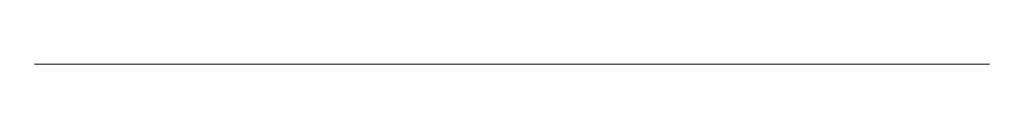
# Model space of a CAD drawing. Units: millimetres. Extents: x 123 to 268, y 0 to 0.
import ezdxf

# ---------------------------------------------------------------- set-up
doc = ezdxf.new("R2010")
doc.units = ezdxf.units.MM
doc.layers.add('M-CONS', color=8, linetype='Continuous', lineweight=13)

msp = doc.modelspace()

# ---------------------------------------------------------------- linework, layer by layer
at = {"layer": 'M-CONS', "extrusion": (0, -1, 0)}
for points in [[(166.51, 83.51, -0.398119), (155.77, 81.11, 0.901298), (131.96, 49.24)], [(130.84, 50.35), (180.43, 0.81, 0.455533), (210.61, 0.81), (260.21, 50.35)], [(259.09, 49.24, 0.901298), (235.27, 81.11, -0.398119), (224.54, 83.51)]]:
    msp.add_lwpolyline(points, format="xyb", dxfattribs=at)
for centre, radius in [((145.52, 63.94), 10), ((195.52, 63.94), 20), ((195.52, 13.94), 10), ((245.52, 63.94), 10)]:
    msp.add_circle(centre, radius, dxfattribs=at)

doc.saveas('drawing.dxf')
